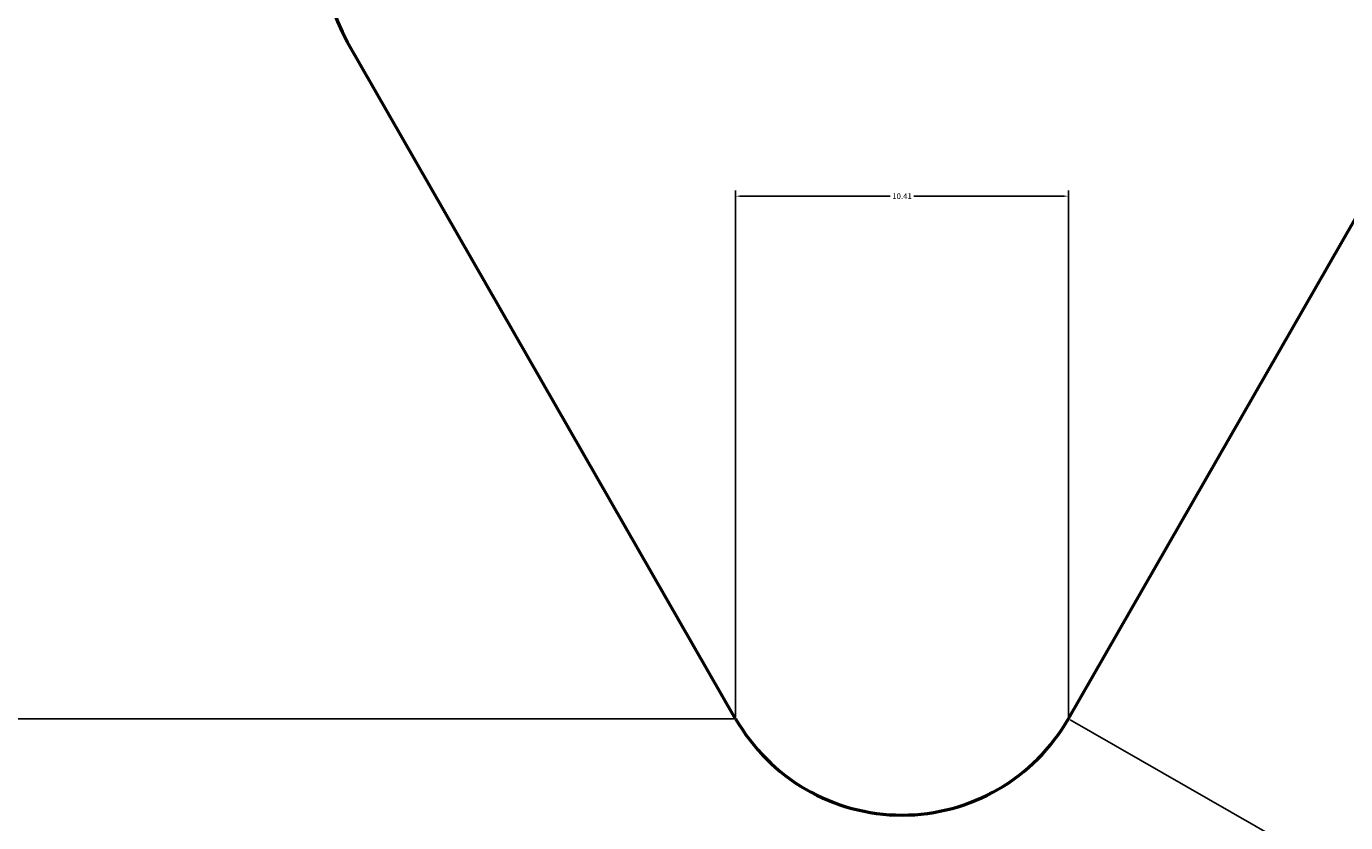
# Model space of a CAD drawing. Units: inches. Extents: x -99 to 284, y -92 to 134.
# Tile 8 of 16: x 5 to 46, y 55 to 80. Entities that reach past the tile are written whole.
import ezdxf

# ---------------------------------------------------------------- set-up
doc = ezdxf.new("R2010")
doc.units = ezdxf.units.IN
doc.header["$MEASUREMENT"] = 0
doc.layers.add('M-DIMS', color=2, linetype='Continuous', lineweight=18)
doc.layers.add('M-OUTL', color=7, linetype='Continuous', lineweight=50)
doc.styles.get("Standard").update_dxf_attribs({"font": 'arial.ttf'})
doc.dimstyles.get("Standard").update_dxf_attribs({"dimtxt": 0.18, "dimasz": 0.18, "dimexe": 0.18, "dimexo": 0.0625, "dimgap": 0.09, "dimtad": 0, "dimtih": 1, "dimtoh": 1, "dimdec": 4, "dimzin": 0, "dimdsep": 46, "dimtxsty": 'Standard', "dimcen": 0.09, "dimadec": 0, "dimazin": 0, "dimtfac": 1, "dimtdec": 4, "dimtofl": 0, "dimtmove": 0, "dimatfit": 3, "dimfxl": 1, "dimtolj": 1, "dimtzin": 0, "dimarcsym": 0})

# ---------------------------------------------------------------- blocks, each defined once
blk = doc.blocks.new('*U1')
for p, q in [((-5.205, -13.52), (-17.34, 7.646)), ((5.205, -13.52), (17.34, 7.646))]:
    blk.add_line(p, q)
for centre, start, end in [((-12.135, 10.63), 100.177, 209.8264), ((12.135, 10.63), 330.1736, 79.823), ((0, -10.536), 209.8264, 330.1736)]:
    blk.add_arc(centre, 6, start, end)
blk = doc.blocks.new('*U2')
at = {"layer": 'M-OUTL', "color": 0, "linetype": 'ByBlock', "lineweight": -2, "transparency": 16777216}
blk.add_blockref('*U1', (31.976, 71.823), dxfattribs=at)
blk = doc.blocks.new('*D9')
at = {"layer": 'Defpoints', "color": 0, "transparency": 16777216}
for p in [(26.771, 58.303), (-73.374, 14.854), (31.976, 14.854)]:
    blk.add_point(p, dxfattribs=at)
at = {"layer": 'M-DIMS', "color": 0, "lineweight": -2, "transparency": 16777216}
for p, q in [((26.709, 58.303), (-73.554, 58.303)), ((-73.374, 58.123), (-73.374, 36.761)), ((-73.374, 15.034), (-73.374, 36.397)), ((31.914, 14.854), (-73.554, 14.854))]:
    blk.add_line(p, q, dxfattribs=at)
at = {"layer": 'M-DIMS', "color": 0, "transparency": 16777216}
for points in [[(-73.404, 58.123), (-73.344, 58.123), (-73.374, 58.303)], [(-73.404, 15.034), (-73.344, 15.034), (-73.374, 14.854)]]:
    blk.add_solid(points, dxfattribs=at)
at = {"layer": 'M-DIMS', "color": 0, "transparency": 16777216, "insert": (-73.374, 36.579), "char_height": 0.18, "attachment_point": 5}
blk.add_mtext('\\A1;43.45', dxfattribs=at)
blk = doc.blocks.new('*D13')
at = {"layer": 'Defpoints', "color": 0, "transparency": 16777216}
for p in [(37.182, 74.653), (26.771, 58.303), (37.182, 58.303)]:
    blk.add_point(p, dxfattribs=at)
at = {"layer": 'M-DIMS', "color": 0, "lineweight": -2, "transparency": 16777216}
for p, q in [((26.771, 58.366), (26.771, 74.833)), ((37.182, 58.366), (37.182, 74.833)), ((26.951, 74.653), (31.609, 74.653)), ((37.002, 74.653), (32.344, 74.653))]:
    blk.add_line(p, q, dxfattribs=at)
at = {"layer": 'M-DIMS', "color": 0, "transparency": 16777216}
for points in [[(26.951, 74.683), (26.951, 74.623), (26.771, 74.653)], [(37.002, 74.683), (37.002, 74.623), (37.182, 74.653)]]:
    blk.add_solid(points, dxfattribs=at)
at = {"layer": 'M-DIMS', "color": 0, "transparency": 16777216, "insert": (31.976, 74.653), "char_height": 0.18, "attachment_point": 5}
blk.add_mtext('\\A1;10.41', dxfattribs=at)
blk = doc.blocks.new('*D14')
at = {"layer": 'Defpoints', "color": 0, "transparency": 16777216}
for p in [(49.317, 79.47), (37.182, 58.303), (51.366, 50.171)]:
    blk.add_point(p, dxfattribs=at)
at = {"layer": 'M-DIMS', "color": 0, "lineweight": -2, "transparency": 16777216}
for p, q in [((49.371, 79.439), (63.657, 71.248)), ((63.412, 71.181), (57.537, 60.935)), ((51.455, 50.327), (57.33, 60.574)), ((37.236, 58.272), (51.522, 50.082))]:
    blk.add_line(p, q, dxfattribs=at)
at = {"layer": 'M-DIMS', "color": 0, "transparency": 16777216}
for points in [[(63.385, 71.196), (63.438, 71.167), (63.501, 71.338)], [(51.429, 50.342), (51.481, 50.312), (51.366, 50.171)]]:
    blk.add_solid(points, dxfattribs=at)
at = {"layer": 'M-DIMS', "color": 0, "transparency": 16777216, "insert": (57.433, 60.754), "char_height": 0.18, "attachment_point": 5}
blk.add_mtext('\\A1;24.4', dxfattribs=at)
blk = doc.blocks.new('*D20')
at = {"layer": 'Defpoints', "color": 0, "transparency": 16777216}
for p in [(-35.23, 65.245), (99.183, -35.537)]:
    blk.add_point(p, dxfattribs=at)
at = {"layer": 'M-DIMS', "color": 0, "lineweight": -2, "transparency": 16777216}
for p, q in [((31.976, 14.764), (31.976, 14.944)), ((31.886, 14.854), (32.066, 14.854)), ((139.507, -65.772), (99.327, -35.645)), ((139.687, -65.772), (139.507, -65.772))]:
    blk.add_line(p, q, dxfattribs=at)
at = {"layer": 'M-DIMS', "color": 0, "transparency": 16777216}
blk.add_solid([(99.345, -35.621), (99.309, -35.669), (99.183, -35.537)], dxfattribs=at)
at = {"layer": 'M-DIMS', "color": 0, "transparency": 16777216, "insert": (140.074, -65.772), "char_height": 0.18, "attachment_point": 5}
blk.add_mtext('\\A1;∅168', dxfattribs=at)
blk = doc.blocks.new('*D22')
at = {"layer": 'Defpoints', "color": 0, "transparency": 16777216}
for p in [(39, 89.203), (31.976, 14.854)]:
    blk.add_point(p, dxfattribs=at)
at = {"layer": 'M-DIMS', "color": 0, "lineweight": -2, "transparency": 16777216}
for p, q in [((43.215, 133.813), (39.017, 89.383)), ((43.395, 133.813), (43.215, 133.813)), ((31.976, 14.764), (31.976, 14.944)), ((31.886, 14.854), (32.066, 14.854))]:
    blk.add_line(p, q, dxfattribs=at)
at = {"layer": 'M-DIMS', "color": 0, "transparency": 16777216}
blk.add_solid([(38.987, 89.385), (39.047, 89.38), (39, 89.203)], dxfattribs=at)
at = {"layer": 'M-DIMS', "color": 0, "transparency": 16777216, "insert": (44.068, 133.813), "char_height": 0.18, "attachment_point": 5}
blk.add_mtext('\\A1;5X R74.68', dxfattribs=at)

msp = doc.modelspace()

# ---------------------------------------------------------------- linework, layer by layer
at = {"layer": 'M-OUTL'}
for radius in [89, 84]:
    msp.add_circle((31.9765, 14.8539), radius, dxfattribs=at)

# ---------------------------------------------------------------- block references
msp.add_blockref('*U2', (0, 0), dxfattribs=at)

# ---------------------------------------------------------------- dimensions: what is measured, and where the dimension line sits
at = {"layer": 'M-DIMS'}
dim = msp.add_radius_dim(center=(31.9765, 14.8539), mpoint=(39.0003, 89.2035), text='5X <>', dimstyle='Standard', override={"dimdec": 2, "dimlfac": 1, "dimrnd": 0, "dimzin": 0, "dimdsep": 46, "dimlunit": 2}, dxfattribs=at)
dim.commit()
dim.dimension.update_dxf_attribs({"geometry": '*D22', "text_midpoint": (44.068, 133.8132), "dimtype": 164})
for base, p1, p2, angle, override, picture, middle in [((51.3659, 50.1711), (49.3168, 79.4697), (37.1817, 58.3032), 240.17365, {"dimdec": 1, "dimlfac": 1, "dimrnd": 0, "dimzin": 0, "dimdsep": 46, "dimlunit": 2}, '*D14', (57.4335, 60.7544)), ((-73.3735, 14.8539), (26.7713, 58.3032), (31.9765, 14.8539), 90, {"dimdec": 2, "dimlfac": 1, "dimrnd": 0, "dimzin": 0, "dimdsep": 46, "dimlunit": 2}, '*D9', (-73.3735, 36.5785))]:
    dim = msp.add_linear_dim(base=base, p1=p1, p2=p2, angle=angle, dimstyle='Standard', override=override, dxfattribs=at)
    dim.commit()
    dim.dimension.update_dxf_attribs({"geometry": picture, "text_midpoint": middle})
dim = msp.add_linear_dim(base=(37.1817, 74.6532), p1=(26.7713, 58.3032), p2=(37.1817, 58.3032), dimstyle='Standard', override={"dimdec": 2, "dimlfac": 1, "dimrnd": 0, "dimzin": 0, "dimdsep": 46, "dimlunit": 2}, dxfattribs=at)
dim.commit()
dim.dimension.update_dxf_attribs({"geometry": '*D13', "text_midpoint": (31.9765, 74.6532)})
dim = msp.add_diameter_dim_2p(p1=(-35.2301, 65.2451), p2=(99.1831, -35.5373), dimstyle='Standard', override={"dimdec": 0, "dimlfac": 1, "dimrnd": 0, "dimzin": 0, "dimdsep": 46, "dimlunit": 2}, dxfattribs=at)
dim.commit()
dim.dimension.update_dxf_attribs({"geometry": '*D20', "text_midpoint": (140.074, -65.772), "dimtype": 163})

doc.saveas('drawing.dxf')
